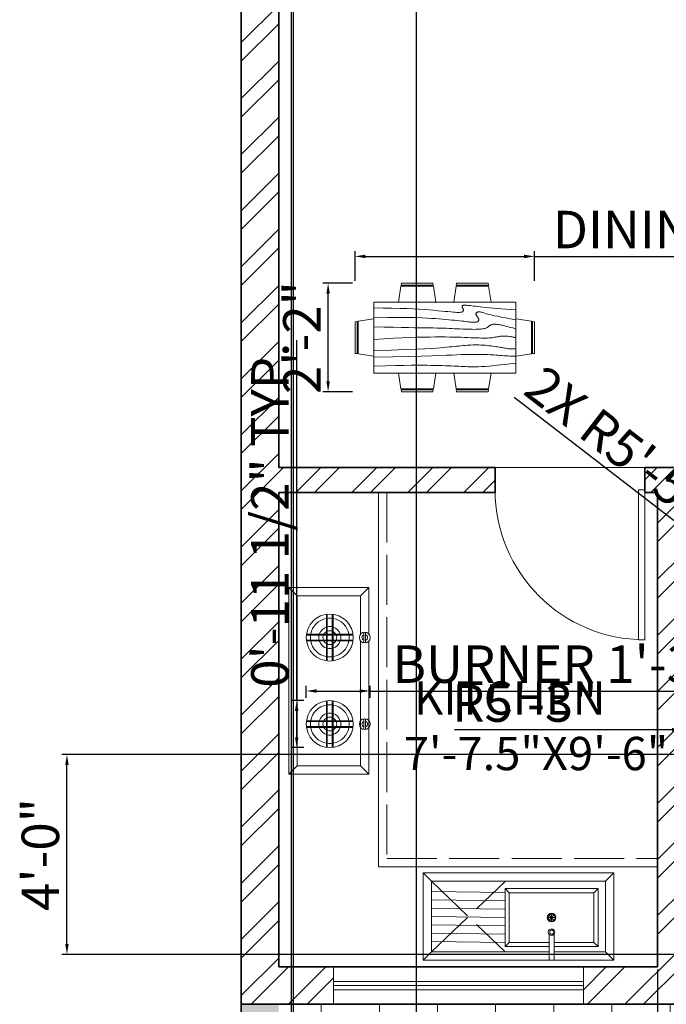
# Model space of a CAD drawing. Units: inches. Extents: x 287 to 905, y 1151 to 2037.
# Tile 2 of 5: x 361 to 516, y 1503 to 1739. Entities that reach past the tile are written whole.
import ezdxf

# ---------------------------------------------------------------- set-up
doc = ezdxf.new("R2010")
doc.units = ezdxf.units.IN
doc.linetypes.add('ACAD_ISO02W100', pattern=[15, 12, -3])
for name, color, linetype, lineweight in [('A-ANNO-DIMS', 2, 'Continuous', 18), ('A-AREA-IDEN', 7, 'Continuous', 18), ('A-DOOR', 4, 'Continuous', 18), ('A-EQPM', 8, 'Continuous', 18), ('A-FLOR-CASE', 8, 'Continuous', 18), ('A-FLOR-CASE-HIDN', 8, 'ACAD_ISO02W100', 13), ('A-FLOR-FIXT', 8, 'Continuous', 18), ('A-FLOR-FIXT-HIDN', 8, 'ACAD_ISO02W100', 13), ('A-FLOR-FIXT-PATT', 9, 'Continuous', 13), ('A-FLOR-PATT', 252, 'Continuous', 13), ('A-FURN', 9, 'Continuous', 18), ('A-WALL', 7, 'Continuous', 35), ('A-WALL-PATT', 252, 'Continuous', 13), ('L-WALL-PATT', 252, 'Continuous', 13)]:
    doc.layers.add(name, color=color, linetype=linetype, lineweight=lineweight)
doc.layers.add('A-GLAZ', color=244, linetype='Continuous', lineweight=18, true_color=0x991b1e)
doc.styles.get("Standard").update_dxf_attribs({"font": 'arial.ttf'})
doc.dimstyles.new('ISO-25', dxfattribs={"dimtxt": 9, "dimasz": 2.5, "dimexe": 1.25, "dimexo": 0.625, "dimtad": 1, "dimlunit": 3, "dimtxsty": 'Standard', "dimcen": 2.5, "dimadec": 0, "dimazin": 0, "dimtfac": 1, "dimtmove": 0, "dimatfit": 3, "dimfxl": 1, "dimarcsym": 0})

# ---------------------------------------------------------------- blocks, each defined once
blk = doc.blocks.new('*U6')
for p, q in [((0, 0), (0, -6)), ((40, 0), (40, -6))]:
    blk.add_line(p, q)
blk.add_lwpolyline([(0, 0), (0, 40), (1.75, 40), (1.75, 0)], close=True)
blk.add_arc((0, 0), 40, 0, 90)
blk = doc.blocks.new('Dining Set - 36 x 72 in.')
for p, q in [((-22.2343, 26.00059), (-23.4847, 17.99762)), ((-22.2304, 26), (-5.7608, 26)), ((-22, 27.5), (-22.1562, 26.50042)), ((-5.8416, 26.5), (-22.1534, 26.5)), ((-22, 27.5), (-6, 27.5)), ((-5.8437, 26.49966), (-6, 27.5)), ((-4.5152, 17.99762), (-5.7655, 25.99926)), ((5.7657, 26.00059), (4.5153, 17.99762)), ((5.7696, 26), (22.2392, 26)), ((6, 27.5), (5.8438, 26.50042)), ((22.1584, 26.5), (5.8466, 26.5)), ((6, 27.5), (22, 27.5)), ((22.1563, 26.49966), (22, 27.5)), ((23.4848, 17.99762), (22.2345, 25.99926)), ((36, 18), (-36, 18)), ((-36, 18), (-36, -18)), ((36, -18), (36, 18)), ((-45.5, 8), (-44.5004, 8.15617)), ((-45.5, 8), (-45.5, -8)), ((-44.5, -8.15843), (-44.5, 8.15338)), ((-44.0006, 8.23428), (-35.9976, 9.48474)), ((-44, 8.23041), (-44, -8.23915)), ((44.0006, 8.23428), (35.9976, 9.48474)), ((44, 8.23041), (44, -8.23915)), ((44.5, -8.15843), (44.5, 8.15338)), ((45.5, 8), (44.5005, 8.15617)), ((45.5, 8), (45.5, -8)), ((-44.4997, -8.15631), (-45.5, -8)), ((-35.9976, -9.48476), (-43.9993, -8.2345)), ((35.9976, -9.48476), (43.9993, -8.2345)), ((44.4997, -8.15631), (45.5, -8)), ((-36, -18), (36, -18)), ((-22.2343, -26.0006), (-23.4847, -17.99762)), ((-4.5152, -17.99762), (-5.7655, -25.99928)), ((5.7657, -26.0006), (4.5153, -17.99762)), ((23.4848, -17.99762), (22.2345, -25.99928)), ((-22.2304, -26), (-5.7608, -26)), ((-22, -27.5), (-22.1562, -26.50044)), ((-5.8416, -26.5), (-22.1534, -26.5)), ((-22, -27.5), (-6, -27.5)), ((-5.8437, -26.49967), (-6, -27.5)), ((5.7696, -26), (22.2392, -26)), ((6, -27.5), (5.8438, -26.50044)), ((22.1584, -26.5), (5.8466, -26.5)), ((6, -27.5), (22, -27.5)), ((22.1563, -26.49967), (22, -27.5))]:
    blk.add_line(p, q)
for points in [[(-36, 15), (-31.1772, 14.97754), (-26.8079, 14.91406), (-22.8538, 14.81543), (-19.276, 14.6875), (-16.0362, 14.53613), (-13.0957, 14.36718), (-10.4159, 14.18652), (-7.9583, 14), (-5.6904, 13.81315), (-3.6035, 13.63021), (-1.6954, 13.45508), (0.0365, 13.29166), (1.5945, 13.14388), (2.9811, 13.01562), (4.1988, 12.9108), (5.25, 12.83333), (6.1393, 12.78613), (6.8802, 12.76823), (7.4883, 12.77767), (7.9792, 12.8125), (8.3685, 12.87077), (8.6719, 12.95052), (8.9049, 13.0498), (9.0833, 13.16666), (9.2205, 13.29899), (9.3216, 13.44401), (9.3895, 13.59879), (9.4271, 13.76041), (9.4373, 13.92594), (9.4232, 14.09245), (9.3875, 14.257), (9.3333, 14.41666), (9.2638, 14.56917), (9.1836, 14.71484), (9.0975, 14.85465), (9.0104, 14.98958), (8.9272, 15.1206), (8.8529, 15.2487), (8.7922, 15.37483), (8.75, 15.5), (8.7305, 15.62467), (8.7344, 15.74739), (8.7617, 15.86621), (8.8125, 15.97916), (8.8867, 16.08431), (8.9844, 16.17968), (9.1055, 16.26334), (9.25, 16.33333), (9.4189, 16.38802), (9.6172, 16.42708), (9.8506, 16.45052), (10.125, 16.45833), (10.4463, 16.45052), (10.8203, 16.42708), (11.2529, 16.38802), (11.75, 16.33333), (12.3184, 16.26318), (12.9694, 16.17838), (13.7151, 16.07991), (14.5677, 15.96875), (15.5395, 15.84586), (16.6426, 15.71224), (17.8893, 15.56884), (19.2917, 15.41666), (20.859, 15.25667), (22.5879, 15.08984), (24.4721, 14.91715), (26.5052, 14.73958), (28.6809, 14.5581), (30.9929, 14.3737), (33.4347, 14.18733), (36, 14)], [(-36, 10), (-28.9766, 10.14274), (-23.1725, 10.20442), (-18.4241, 10.19775), (-14.5677, 10.13541), (-11.4399, 10.03011), (-8.877, 9.89453), (-6.7154, 9.74137), (-4.7917, 9.58333), (-2.9698, 9.43082), (-1.2246, 9.28515), (0.4415, 9.14534), (2.026, 9.01041), (3.5266, 8.87939), (4.9408, 8.7513), (6.266, 8.62516), (7.5, 8.5), (8.6411, 8.37549), (9.6914, 8.2539), (10.6538, 8.13818), (11.5312, 8.03125), (12.3267, 7.93603), (13.043, 7.85547), (13.6831, 7.79248), (14.25, 7.75), (14.7471, 7.7303), (15.1797, 7.73307), (15.5537, 7.75732), (15.875, 7.80208), (16.1494, 7.86637), (16.3828, 7.94922), (16.5811, 8.04964), (16.75, 8.16666), (16.8944, 8.29915), (17.0143, 8.44531), (17.1089, 8.60319), (17.1771, 8.77083), (17.218, 8.94629), (17.2305, 9.1276), (17.2137, 9.31282), (17.1667, 9.5), (17.0895, 9.6875), (16.987, 9.875), (16.8649, 10.0625), (16.7292, 10.25), (16.5856, 10.4375), (16.4401, 10.625), (16.2985, 10.8125), (16.1667, 11), (16.05, 11.18733), (15.9518, 11.3737), (15.8752, 11.5581), (15.8229, 11.73958), (15.798, 11.91715), (15.8034, 12.08984), (15.842, 12.25667), (15.9167, 12.41666), (16.0295, 12.56836), (16.1784, 12.70833), (16.3605, 12.83268), (16.5729, 12.9375), (16.8127, 13.01888), (17.0768, 13.07291), (17.3625, 13.0957), (17.6667, 13.08333), (17.9894, 13.03312), (18.3418, 12.94726), (18.7382, 12.82918), (19.1927, 12.68229), (19.7195, 12.51001), (20.3327, 12.31575), (21.0465, 12.10294), (21.875, 11.875), (22.8357, 11.63354), (23.959, 11.37304), (25.2786, 11.08618), (26.8282, 10.76562), (28.6414, 10.40405), (30.752, 9.99414), (33.1936, 9.52856), (36, 9)], [(-36, 5.5), (-30.7157, 5.3348), (-26.069, 5.20963), (-21.9946, 5.11767), (-18.4271, 5.05208), (-15.3009, 5.00602), (-12.5508, 4.97265), (-10.1112, 4.94515), (-7.9167, 4.91666), (-5.909, 4.88167), (-4.0586, 4.83984), (-2.3429, 4.79215), (-0.7396, 4.73958), (0.7739, 4.6831), (2.22, 4.6237), (3.6213, 4.56233), (5, 4.5), (6.373, 4.43782), (7.7344, 4.3776), (9.0723, 4.32129), (10.375, 4.27083), (11.6309, 4.22819), (12.8281, 4.19531), (13.9551, 4.17415), (15, 4.16666), (15.954, 4.17448), (16.819, 4.19791), (17.6001, 4.23698), (18.3021, 4.29166), (18.9299, 4.36198), (19.4883, 4.44791), (19.9823, 4.54948), (20.4167, 4.66666), (20.7969, 4.79899), (21.1302, 4.94401), (21.4245, 5.09879), (21.6875, 5.26041), (21.9271, 5.42594), (22.1511, 5.59245), (22.3672, 5.757), (22.5834, 5.91666), (22.8065, 6.06868), (23.0404, 6.21093), (23.2879, 6.34147), (23.5521, 6.45833), (23.8358, 6.55957), (24.142, 6.64323), (24.4735, 6.70735), (24.8334, 6.75), (25.2235, 6.76969), (25.642, 6.76692), (26.0858, 6.74267), (26.5521, 6.69791), (27.0379, 6.63362), (27.5404, 6.55078), (28.0565, 6.45036), (28.5834, 6.33333), (29.1242, 6.19987), (29.7071, 6.04687), (30.3661, 5.87044), (31.1354, 5.66666), (32.0493, 5.43164), (33.142, 5.16146), (34.4475, 4.85221), (36, 4.5)], [(-36, -1), (-30.7915, -0.6591), (-26.0195, -0.38216), (-21.6519, -0.16284), (-17.6563, 0.00521), (-14.0005, 0.12833), (-10.6523, 0.21289), (-7.5796, 0.26522), (-4.75, 0.29166), (-2.134, 0.29793), (0.2878, 0.28711), (2.5317, 0.26163), (4.6146, 0.22396), (6.5529, 0.17651), (8.3633, 0.12174), (10.0623, 0.06209), (11.6667, 0), (13.1899, -0.06201), (14.6341, -0.1211), (15.9982, -0.17432), (17.2813, -0.21875), (18.4823, -0.25147), (19.6003, -0.26953), (20.6343, -0.27002), (21.5834, -0.25), (22.4481, -0.20768), (23.2357, -0.14584), (23.9549, -0.06836), (24.6146, 0.02083), (25.2235, 0.11784), (25.7904, 0.21875), (26.3241, 0.31966), (26.8334, 0.41666), (27.3265, 0.50618), (27.8099, 0.58593), (28.2894, 0.65397), (28.7709, 0.70833), (29.2601, 0.74707), (29.763, 0.76823), (30.2855, 0.76985), (30.8334, 0.75), (31.4088, 0.70784), (31.9994, 0.64713), (32.589, 0.57275), (33.1615, 0.48958), (33.7008, 0.4025), (34.1908, 0.3164), (34.6153, 0.23616), (34.9584, 0.16666), (35.2099, 0.11165), (35.3848, 0.07031), (35.504, 0.04069), (35.5886, 0.02083), (35.6594, 0.00879), (35.7377, 0.0026), (35.8442, 0.00032), (36, 0)], [(-36, -6.5), (-27.1843, -6.31267), (-20.084, -6.1263), (-14.469, -5.9419), (-10.1094, -5.76042), (-6.7752, -5.58285), (-4.2363, -5.41016), (-2.2629, -5.24333), (-0.625, -5.08334), (0.8708, -4.93099), (2.2715, -4.78646), (3.5872, -4.64974), (4.8281, -4.52084), (6.0046, -4.39974), (7.127, -4.28646), (8.2053, -4.18099), (9.25, -4.08334), (10.2705, -3.99382), (11.2734, -3.91407), (12.2647, -3.84603), (13.25, -3.79167), (14.2354, -3.75293), (15.2266, -3.73177), (16.2295, -3.73015), (17.25, -3.75), (18.2912, -3.79248), (19.3451, -3.85547), (20.4009, -3.93604), (21.4479, -4.03125), (22.4754, -4.13819), (23.4727, -4.25391), (24.4289, -4.37549), (25.3334, -4.5), (26.1785, -4.62492), (26.9694, -4.74935), (27.7145, -4.87281), (28.4219, -4.99479), (29.1, -5.11483), (29.7572, -5.23242), (30.4016, -5.34709), (31.0417, -5.45834), (31.6837, -5.56437), (32.3262, -5.65821), (32.9658, -5.73153), (33.599, -5.77604), (34.2224, -5.78345), (34.8327, -5.74545), (35.4264, -5.65373), (36, -5.5)], [(-36, -10), (-26.4022, -9.81299), (-18.4675, -9.62891), (-11.9839, -9.45069), (-6.7396, -9.28125), (-2.5226, -9.12354), (0.8789, -8.98047), (3.6769, -8.85498), (6.0833, -8.75), (8.2767, -8.66765), (10.3021, -8.60677), (12.1712, -8.56543), (13.8958, -8.54167), (15.4876, -8.53353), (16.9583, -8.53907), (18.3197, -8.55632), (19.5834, -8.58334), (20.7616, -8.61841), (21.8685, -8.66081), (22.9188, -8.71004), (23.9271, -8.76563), (24.9081, -8.82707), (25.8763, -8.89388), (26.8465, -8.96558), (27.8334, -9.04167), (28.8474, -9.12118), (29.8828, -9.20117), (30.93, -9.27824), (31.9792, -9.34896), (33.0205, -9.40991), (34.0443, -9.45768), (35.0407, -9.48885), (36, -9.5)], [(-36, -14.5), (-30.0881, -14.33513), (-25.0332, -14.21224), (-20.7312, -14.12647), (-17.0781, -14.07292), (-13.97, -14.04671), (-11.3027, -14.04297), (-8.9724, -14.05681), (-6.875, -14.08334), (-4.9224, -14.11833), (-3.0905, -14.16016), (-1.3709, -14.20785), (0.2448, -14.26042), (1.7647, -14.3169), (3.1973, -14.3763), (4.5507, -14.43767), (5.8333, -14.5), (7.0554, -14.5621), (8.235, -14.62175), (9.3922, -14.67652), (10.5469, -14.72396), (11.7192, -14.76164), (12.929, -14.78711), (14.1965, -14.79794), (15.5417, -14.79167), (16.9933, -14.76424), (18.6152, -14.70508), (20.4804, -14.60197), (22.6615, -14.44271), (25.2312, -14.21509), (28.2624, -13.9069), (31.8277, -13.50594), (36, -13)]]:
    blk.add_lwpolyline(points)
blk = doc.blocks.new('WIN-60IN')
for p, q in [((-1, 30), (-1, -30)), ((0, 30), (0, -30)), ((1, 30), (1, -30))]:
    blk.add_line(p, q)
blk.add_lwpolyline([(-4.5, 30), (4.5, 30), (4.5, -30), (-4.5, -30)], close=True)
blk = doc.blocks.new('COOKTOP-BURNER-WITH-CONTROL')
for p, q in [((-0.8, 5.6), (-0.8, -5.6)), ((-0.6, 5.62), (-0.6, 0.8)), ((0.6, 5.62), (0.6, 0.8)), ((0.8, 5.6), (0.8, -5.6)), ((-5.62, 0.6), (-0.8, 0.6)), ((-5.6, 0.8), (5.6, 0.8)), ((-0.6, 0.6), (-0.6, -0.6)), ((-0.6, 0.6), (0.6, 0.6)), ((0.6, 0.6), (0.6, -0.6)), ((0.8, 0.6), (5.62, 0.6)), ((8.19, 1.27), (8.19, -1.27)), ((8.59, 1.27), (8.59, -1.27)), ((-5.62, -0.6), (-0.8, -0.6)), ((-5.6, -0.8), (5.6, -0.8)), ((-0.6, -0.6), (0.6, -0.6)), ((-0.6, -0.8), (-0.6, -5.62)), ((0.6, -0.8), (0.6, -5.62)), ((0.8, -0.6), (5.62, -0.6))]:
    blk.add_line(p, q)
for centre, radius in [((0, 0), 5.65), ((8.39, 0), 1.29)]:
    blk.add_circle(centre, radius)
for centre, radius, start, end in [((0, 0), 4.65, 99.901, 170.099), ((0, 0), 2.65, 107.5531, 162.4469), ((0, 0), 4.65, 82.5905, 97.4095), ((0, 0), 2.65, 76.927, 103.073), ((0, 0), 4.65, 9.901, 80.099), ((0, 0), 2.65, 17.5531, 72.4469), ((0, 0), 4.65, 172.5905, 187.4095), ((0, 0), 2.65, 166.927, 193.073), ((0, 0), 1.65, 158.7117, 201.2883), ((0, 0), 1.65, 118.9523, 151.0477), ((0, 0), 1.65, 68.7117, 111.2883), ((0, 0), 1.65, 28.9523, 61.0477), ((0, 0), 1.65, 338.7117, 21.2883), ((0, 0), 2.65, 346.927, 13.073), ((0, 0), 4.65, 352.5905, 7.4095), ((8.39, 0), 0.687, 106.9364, 253.0636), ((8.39, 0), 0.687, 286.9364, 73.0636), ((0, 0), 4.65, 189.901, 260.099), ((0, 0), 2.65, 197.5531, 252.4469), ((0, 0), 1.65, 208.9523, 241.0477), ((0, 0), 1.65, 248.7117, 291.2883), ((0, 0), 4.65, 279.901, 350.099), ((0, 0), 2.65, 287.5531, 342.4469), ((0, 0), 1.65, 298.9523, 331.0477), ((0, 0), 2.65, 256.927, 283.073), ((0, 0), 4.65, 262.5905, 277.4095)]:
    blk.add_arc(centre, radius, start, end)
blk = doc.blocks.new('*D26')
at = {"layer": 'A-ANNO-DIMS', "color": 0, "lineweight": -2, "transparency": 16777216}
for p, q in [((429.49, 1576.45), (429.49, 1579.37)), ((444.82, 1576.45), (444.82, 1579.37)), ((431.99, 1578.12), (442.32, 1578.12)), ((444.82, 1578.12), (580.58, 1578.12))]:
    blk.add_line(p, q, dxfattribs=at)
at = {"layer": 'A-ANNO-DIMS', "color": 0, "transparency": 16777216}
for points in [[(431.99, 1578.54), (431.99, 1577.71), (429.49, 1578.12)], [(442.32, 1578.54), (442.32, 1577.71), (444.82, 1578.12)]]:
    blk.add_solid(points, dxfattribs=at)
at = {"layer": 'Defpoints', "color": 0, "transparency": 16777216}
for p in [(429.49, 1575.83), (444.82, 1578.12), (444.82, 1575.83)]:
    blk.add_point(p, dxfattribs=at)
at = {"layer": 'A-ANNO-DIMS', "color": 0, "transparency": 16777216, "insert": (513.95, 1583.41), "char_height": 9, "attachment_point": 5}
blk.add_mtext('BURNER 1\'-3 1/2" TYP.', dxfattribs=at)
blk = doc.blocks.new('*D27')
at = {"layer": 'A-ANNO-DIMS', "color": 0, "lineweight": -2, "transparency": 16777216}
for p, q in [((427.19, 1575.83), (427.19, 1662.4)), ((428.86, 1575.83), (425.94, 1575.83)), ((427.19, 1567.02), (427.19, 1573.33)), ((428.86, 1564.52), (425.94, 1564.52))]:
    blk.add_line(p, q, dxfattribs=at)
at = {"layer": 'A-ANNO-DIMS', "color": 0, "transparency": 16777216}
for points in [[(426.77, 1573.33), (427.6, 1573.33), (427.19, 1575.83)], [(426.77, 1567.02), (427.6, 1567.02), (427.19, 1564.52)]]:
    blk.add_solid(points, dxfattribs=at)
at = {"layer": 'Defpoints', "color": 0, "transparency": 16777216}
for p in [(427.19, 1575.83), (429.49, 1575.83), (429.49, 1564.52)]:
    blk.add_point(p, dxfattribs=at)
at = {"layer": 'A-ANNO-DIMS', "color": 0, "transparency": 16777216, "insert": (421.91, 1620.36), "char_height": 9, "attachment_point": 5, "rotation": 90}
blk.add_mtext('0\'-11 1/2" TYP.', dxfattribs=at)
blk = doc.blocks.new('*D28')
at = {"layer": 'A-ANNO-DIMS', "color": 0, "lineweight": -2, "transparency": 16777216}
for p, q in [((441.2, 1676.71), (441.2, 1683.81)), ((443.7, 1682.56), (481.83, 1682.56)), ((484.33, 1676.71), (484.33, 1683.81)), ((484.33, 1682.56), (587, 1682.56))]:
    blk.add_line(p, q, dxfattribs=at)
at = {"layer": 'A-ANNO-DIMS', "color": 0, "transparency": 16777216}
for points in [[(443.7, 1682.97), (443.7, 1682.14), (441.2, 1682.56)], [(481.83, 1682.97), (481.83, 1682.14), (484.33, 1682.56)]]:
    blk.add_solid(points, dxfattribs=at)
at = {"layer": 'Defpoints', "color": 0, "transparency": 16777216}
for p in [(484.33, 1682.56), (441.2, 1676.09), (484.33, 1676.09)]:
    blk.add_point(p, dxfattribs=at)
at = {"layer": 'A-ANNO-DIMS', "color": 0, "transparency": 16777216, "insert": (536.92, 1687.84), "char_height": 9, "attachment_point": 5}
blk.add_mtext('DINING SET 3\'-7"', dxfattribs=at)
blk = doc.blocks.new('*D29')
at = {"layer": 'A-ANNO-DIMS', "color": 0, "lineweight": -2, "transparency": 16777216}
for p, q in [((440.58, 1676.09), (433.48, 1676.09)), ((434.73, 1652.52), (434.73, 1673.59)), ((440.58, 1650.02), (433.48, 1650.02))]:
    blk.add_line(p, q, dxfattribs=at)
at = {"layer": 'A-ANNO-DIMS', "color": 0, "transparency": 16777216}
for points in [[(434.32, 1673.59), (435.15, 1673.59), (434.73, 1676.09)], [(434.32, 1652.52), (435.15, 1652.52), (434.73, 1650.02)]]:
    blk.add_solid(points, dxfattribs=at)
at = {"layer": 'Defpoints', "color": 0, "transparency": 16777216}
for p in [(434.73, 1676.09), (441.2, 1676.09), (441.2, 1650.02)]:
    blk.add_point(p, dxfattribs=at)
at = {"layer": 'A-ANNO-DIMS', "color": 0, "transparency": 16777216, "insert": (429.59, 1663.05), "char_height": 9, "attachment_point": 5, "rotation": 90}
blk.add_mtext('2\'-2"', dxfattribs=at)
blk = doc.blocks.new('*D32')
at = {"layer": 'A-ANNO-DIMS', "color": 0, "lineweight": -2, "transparency": 16777216}
for p, q in [((426.39, 1284.46), (426.39, 2019.96)), ((428.89, 2018.71), (564.36, 2018.71)), ((566.86, 1284.46), (566.86, 2019.96))]:
    blk.add_line(p, q, dxfattribs=at)
at = {"layer": 'A-ANNO-DIMS', "color": 0, "transparency": 16777216}
for points in [[(428.89, 2019.12), (428.89, 2018.29), (426.39, 2018.71)], [(564.36, 2019.12), (564.36, 2018.29), (566.86, 2018.71)]]:
    blk.add_solid(points, dxfattribs=at)
at = {"layer": 'Defpoints', "color": 0, "transparency": 16777216}
for p in [(566.86, 2018.71), (426.39, 1283.83), (566.86, 1283.83)]:
    blk.add_point(p, dxfattribs=at)
at = {"layer": 'A-ANNO-DIMS', "color": 0, "transparency": 16777216, "insert": (496.62, 2023.99), "char_height": 9, "attachment_point": 5}
blk.add_mtext('11\'-8 1/2"', dxfattribs=at)
blk = doc.blocks.new('*D35')
at = {"layer": 'A-ANNO-DIMS', "color": 0, "lineweight": -2, "transparency": 16777216}
for p, q in [((651.73, 1562.83), (370.73, 1562.83)), ((371.98, 1517.33), (371.98, 1560.33)), ((651.73, 1514.83), (370.73, 1514.83))]:
    blk.add_line(p, q, dxfattribs=at)
at = {"layer": 'A-ANNO-DIMS', "color": 0, "transparency": 16777216}
for points in [[(371.57, 1560.33), (372.4, 1560.33), (371.98, 1562.83)], [(371.57, 1517.33), (372.4, 1517.33), (371.98, 1514.83)]]:
    blk.add_solid(points, dxfattribs=at)
at = {"layer": 'Defpoints', "color": 0, "transparency": 16777216}
for p in [(371.98, 1562.83), (652.36, 1562.83), (652.36, 1514.83)]:
    blk.add_point(p, dxfattribs=at)
at = {"layer": 'A-ANNO-DIMS', "color": 0, "transparency": 16777216, "insert": (366.76, 1538.83), "char_height": 9, "attachment_point": 5, "rotation": 90}
blk.add_mtext('4\'-0"', dxfattribs=at)
blk = doc.blocks.new('*D36')
at = {"layer": 'A-ANNO-DIMS', "color": 0, "lineweight": -2, "transparency": 16777216}
for p, q in [((513.86, 1511.21), (513.86, 1157.65)), ((519.86, 1511.21), (519.86, 1157.65)), ((511.36, 1158.9), (508.86, 1158.9)), ((513.86, 1158.9), (519.86, 1158.9)), ((522.36, 1158.9), (550.03, 1158.9))]:
    blk.add_line(p, q, dxfattribs=at)
at = {"layer": 'A-ANNO-DIMS', "color": 0, "transparency": 16777216}
for points in [[(511.36, 1159.32), (511.36, 1158.49), (513.86, 1158.9)], [(522.36, 1159.32), (522.36, 1158.49), (519.86, 1158.9)]]:
    blk.add_solid(points, dxfattribs=at)
at = {"layer": 'Defpoints', "color": 0, "transparency": 16777216}
for p in [(513.86, 1511.83), (519.86, 1511.83), (519.86, 1158.9)]:
    blk.add_point(p, dxfattribs=at)
at = {"layer": 'A-ANNO-DIMS', "color": 0, "transparency": 16777216, "insert": (537.44, 1164.12), "char_height": 9, "attachment_point": 5}
blk.add_mtext('0\'-6"', dxfattribs=at)
blk = doc.blocks.new('*D38')
at = {"layer": 'A-ANNO-DIMS', "color": 0, "lineweight": -2, "transparency": 16777216}
for p, q in [((425.86, 1913.21), (425.86, 1157.65)), ((455.86, 1913.21), (455.86, 1157.65)), ((428.36, 1158.9), (453.36, 1158.9))]:
    blk.add_line(p, q, dxfattribs=at)
at = {"layer": 'A-ANNO-DIMS', "color": 0, "transparency": 16777216}
for points in [[(428.36, 1159.32), (428.36, 1158.49), (425.86, 1158.9)], [(453.36, 1159.32), (453.36, 1158.49), (455.86, 1158.9)]]:
    blk.add_solid(points, dxfattribs=at)
at = {"layer": 'Defpoints', "color": 0, "transparency": 16777216}
for p in [(425.86, 1913.83), (455.86, 1913.83), (455.86, 1158.9)]:
    blk.add_point(p, dxfattribs=at)
at = {"layer": 'A-ANNO-DIMS', "color": 0, "transparency": 16777216, "insert": (440.86, 1164.12), "char_height": 9, "attachment_point": 5}
blk.add_mtext('2\'-6"', dxfattribs=at)
blk = doc.blocks.new('*D41')
at = {"layer": 'A-ANNO-DIMS', "color": 0, "lineweight": -2, "transparency": 16777216}
for p, q in [((479.4, 1648.76), (529.44, 1610.15)), ((582.98, 1568.83), (531.42, 1608.62))]:
    blk.add_line(p, q, dxfattribs=at)
at = {"layer": 'A-ANNO-DIMS', "color": 0, "transparency": 16777216}
blk.add_solid([(529.7, 1610.48), (529.19, 1609.82), (531.42, 1608.62)], dxfattribs=at)
at = {"layer": 'Defpoints', "color": 0, "transparency": 16777216}
for p in [(531.42, 1608.62), (582.98, 1568.83)]:
    blk.add_point(p, dxfattribs=at)
at = {"layer": 'A-ANNO-DIMS', "color": 0, "transparency": 16777216, "insert": (503.67, 1636.62), "char_height": 9, "attachment_point": 5, "rotation": 322.3456}
blk.add_mtext('2X R5\'-5"', dxfattribs=at)
blk = doc.blocks.new('*D42')
at = {"layer": 'A-ANNO-DIMS', "color": 0, "lineweight": -2, "transparency": 16777216}
for p, q in [((465.09, 1568.83), (517.36, 1568.83)), ((582.98, 1568.83), (519.86, 1568.83))]:
    blk.add_line(p, q, dxfattribs=at)
at = {"layer": 'A-ANNO-DIMS', "color": 0, "transparency": 16777216}
blk.add_solid([(517.36, 1569.25), (517.36, 1568.42), (519.86, 1568.83)], dxfattribs=at)
at = {"layer": 'Defpoints', "color": 0, "transparency": 16777216}
for p in [(519.86, 1568.83), (582.98, 1568.83)]:
    blk.add_point(p, dxfattribs=at)
at = {"layer": 'A-ANNO-DIMS', "color": 0, "transparency": 16777216, "insert": (481.98, 1574.06), "char_height": 9, "attachment_point": 5, "rotation": 0.0002}
blk.add_mtext('R5\'-3"', dxfattribs=at)

msp = doc.modelspace()

# ---------------------------------------------------------------- hatches: boundary and pattern name
at = {"layer": 'A-FLOR-FIXT-PATT'}
h = msp.add_hatch(dxfattribs=at)
h.set_pattern_fill('ANSI31', color=256, scale=0.6300798, angle=134.1764, style=0)
h.paths.add_polyline_path([(459.583, 1517.736), (477.272, 1517.482), (477.272, 1529.883), (459.583, 1530.137)])
at = {"layer": 'A-FLOR-PATT'}
h = msp.add_hatch(dxfattribs=at)
h.set_pattern_fill('ANGLE', color=256, scale=2)
h.set_pattern_definition([(0, (0, 0), (0, 13.97), [10.16, -3.81]), (90, (0, 0), (-13.97, 9e-16), [10.16, -3.81])])
h.paths.add_polyline_path([(588.313, 1502.833), (422.857, 1502.833), (422.857, 1283.833), (588.313, 1283.833)])
h.paths.add_polyline_path([(486.188, 1389.005), (563.901, 1389.005), (563.901, 1418.856), (486.188, 1418.856)], flags=24)
at = {"layer": 'A-WALL-PATT'}
h = msp.add_hatch(dxfattribs=at)
h.set_pattern_fill('ANSI32', color=256)
h.paths.add_polyline_path([(422.857, 1775.833), (561.857, 1775.833), (561.857, 1781.833), (568.629, 1788.605), (564.387, 1792.848), (553.372, 1781.833), (422.857, 1781.833), (422.857, 1913.833), (425.857, 1913.833), (425.857, 1919.833), (422.857, 1919.833), (422.857, 1967.833), (452.78, 1967.833), (452.78, 1976.833), (413.857, 1976.833), (413.857, 1502.833), (436.063, 1502.833), (436.063, 1511.833), (422.857, 1511.833), (422.857, 1625.833), (474.857, 1625.833), (474.857, 1631.833), (422.857, 1631.833)])
h = msp.add_hatch(dxfattribs=at)
h.set_pattern_fill('ANSI32', color=256)
h.paths.add_polyline_path([(604.357, 1511.833), (519.857, 1511.833), (519.857, 1625.833), (607.357, 1625.833), (607.357, 1631.833), (510.857, 1631.833), (510.857, 1625.833), (513.857, 1625.833), (513.857, 1511.833), (496.063, 1511.833), (496.063, 1502.833), (604.357, 1502.833)])
h.paths.add_polyline_path([(652.357, 1511.833), (652.357, 1514.833), (643.357, 1514.833), (643.357, 1511.833), (640.357, 1511.833), (640.357, 1505.833), (643.357, 1505.833), (643.357, 1370.833), (690.607, 1370.833), (690.607, 1379.833), (652.357, 1379.833)])
h.paths.add_polyline_path([(797.857, 1582.055), (788.857, 1582.055), (788.857, 1571.833), (703.357, 1571.833), (703.357, 1574.833), (697.357, 1574.833), (697.357, 1571.833), (652.357, 1571.833), (652.357, 1574.833), (646.357, 1574.833), (646.357, 1562.833), (652.357, 1562.833), (652.357, 1565.833), (788.857, 1565.833), (788.857, 1379.833), (750.607, 1379.833), (750.607, 1370.833), (797.857, 1370.833)])
h.paths.add_polyline_path([(797.857, 1673.833), (788.857, 1673.833), (788.857, 1631.833), (685.357, 1631.833), (685.357, 1625.833), (697.357, 1625.833), (697.357, 1604.833), (703.357, 1604.833), (703.357, 1625.833), (788.857, 1625.833), (788.857, 1603.055), (797.857, 1603.055)])
h.paths.add_polyline_path([(797.857, 1976.833), (751.357, 1976.833), (751.357, 1967.833), (788.857, 1967.833), (788.857, 1919.833), (785.857, 1919.833), (785.857, 1913.833), (788.857, 1913.833), (788.857, 1781.833), (654.342, 1781.833), (643.328, 1792.848), (639.085, 1788.605), (645.857, 1781.833), (645.857, 1775.833), (646.357, 1775.833), (646.357, 1772.833), (652.357, 1772.833), (652.357, 1775.833), (788.857, 1775.833), (788.857, 1733.833), (797.857, 1733.833)])
h.paths.add_polyline_path([(755.857, 1919.833), (692.857, 1919.833), (692.857, 1967.833), (730.357, 1967.833), (730.357, 1976.833), (473.78, 1976.833), (473.78, 1967.833), (518.857, 1967.833), (518.857, 1919.833), (455.857, 1919.833), (455.857, 1913.833), (567.857, 1913.833), (567.857, 1919.833), (524.857, 1919.833), (524.857, 1967.833), (686.857, 1967.833), (686.857, 1919.833), (639.857, 1919.833), (639.857, 1913.833), (755.857, 1913.833)])
h.paths.add_polyline_path([(606.857, 1913.833), (609.857, 1913.833), (609.857, 1919.833), (597.857, 1919.833), (597.857, 1913.833), (600.857, 1913.833), (600.857, 1829.319), (589.842, 1818.304), (594.085, 1814.061), (600.857, 1820.833), (600.857, 1781.833), (597.857, 1781.833), (597.857, 1775.833), (609.857, 1775.833), (609.857, 1781.833), (606.857, 1781.833), (606.857, 1820.833), (613.629, 1814.061), (617.872, 1818.304), (606.857, 1829.319)])
h.paths.add_polyline_path([(652.357, 1736.833), (646.357, 1736.833), (646.357, 1631.833), (643.357, 1631.833), (643.357, 1625.833), (646.357, 1625.833), (646.357, 1604.833), (652.357, 1604.833), (652.357, 1625.833), (655.357, 1625.833), (655.357, 1631.833), (652.357, 1631.833)])
at = {"layer": 'L-WALL-PATT'}
h = msp.add_hatch(color=256, dxfattribs=at)
h.dxf.hatch_style = 1
h.paths.add_polyline_path([(422.857, 1502.833), (413.857, 1502.833), (413.857, 1277.833), (426.388, 1277.833), (426.388, 1283.833), (422.857, 1283.833)])
h.paths.add_polyline_path([(644.857, 1283.833), (635.857, 1283.833), (635.857, 1277.833), (644.857, 1277.833)])
h.paths.add_polyline_path([(575.857, 1283.833), (566.857, 1283.833), (566.857, 1277.833), (575.857, 1277.833)])

# ---------------------------------------------------------------- linework, layer by layer
at = {"layer": 'A-DOOR'}
msp.add_line((510.857, 1631.833), (474.857, 1631.833), dxfattribs=at)
at = {"layer": 'A-EQPM'}
for p, q in [((427.324, 1601.014), (425.324, 1603.014)), ((442.531, 1601.014), (444.531, 1603.014)), ((427.324, 1560.115), (425.324, 1558.115)), ((442.531, 1560.115), (444.531, 1558.115))]:
    msp.add_line(p, q, dxfattribs=at)
for points in [[(444.531, 1590.148), (444.531, 1558.115), (425.324, 1558.115), (425.324, 1603.014), (444.531, 1603.014), (444.531, 1591.767)], [(442.531, 1590.148), (442.531, 1560.115), (427.324, 1560.115), (427.324, 1601.014), (442.531, 1601.014), (442.531, 1591.767)]]:
    msp.add_lwpolyline(points, dxfattribs=at)
at = {"layer": 'A-FLOR-CASE'}
for p, q in [((446.857, 1625.833), (446.857, 1535.833)), ((446.857, 1535.833), (513.857, 1535.833))]:
    msp.add_line(p, q, dxfattribs=at)
at = {"layer": 'A-FLOR-CASE-HIDN'}
for p, q in [((448.857, 1625.833), (448.857, 1537.833)), ((448.857, 1537.833), (513.857, 1537.833))]:
    msp.add_line(p, q, dxfattribs=at)
at = {"layer": 'A-FLOR-FIXT'}
for p, q in [((459.583, 1532.456), (457.583, 1534.456)), ((501.344, 1532.456), (503.344, 1534.456)), ((478.272, 1529.649), (477.272, 1530.649)), ((498.6, 1529.649), (499.6, 1530.649)), ((489.162, 1522.928), (487.71, 1524.437)), ((487.722, 1522.917), (489.15, 1524.448)), ((488.436, 1524.729), (488.436, 1522.636)), ((487.389, 1523.683), (489.483, 1523.683)), ((487.836, 1513.418), (487.836, 1519.657)), ((489.036, 1513.418), (489.036, 1519.657)), ((478.272, 1517.716), (477.272, 1516.716)), ((498.6, 1517.716), (499.6, 1516.716)), ((459.583, 1515.418), (457.583, 1513.418)), ((501.344, 1515.418), (503.344, 1513.418))]:
    msp.add_line(p, q, dxfattribs=at)
msp.add_lwpolyline([(457.583, 1534.456), (503.344, 1534.456), (503.344, 1513.418), (457.583, 1513.418)], close=True, dxfattribs=at)
for points in [[(487.836, 1515.418), (459.583, 1515.418), (459.583, 1532.456), (501.344, 1532.456), (501.344, 1515.418), (489.036, 1515.418)], [(489.036, 1516.716), (499.6, 1516.716), (499.6, 1530.649), (477.272, 1530.649), (477.272, 1516.716), (487.836, 1516.716)], [(489.036, 1517.716), (498.6, 1517.716), (498.6, 1529.649), (478.272, 1529.649), (478.272, 1517.716), (487.836, 1517.716)]]:
    msp.add_lwpolyline(points, dxfattribs=at)
for centre, radius in [((488.436, 1523.683), 1.047), ((488.436, 1523.683), 0.847), ((488.436, 1520.176), 0.793), ((488.436, 1520.176), 0.493)]:
    msp.add_circle(centre, radius, dxfattribs=at)
at = {"layer": 'A-FLOR-FIXT-HIDN'}
for p, q in [((459.583, 1532.456), (477.272, 1515.418)), ((459.583, 1515.418), (477.336, 1532.456))]:
    msp.add_line(p, q, dxfattribs=at)
at = {"layer": 'A-WALL'}
for p, q in [((413.857, 1976.833), (413.857, 1277.833)), ((422.857, 1775.833), (422.857, 1631.833)), ((422.857, 1631.833), (474.857, 1631.833)), ((474.857, 1625.833), (474.857, 1631.833)), ((510.857, 1625.833), (510.857, 1631.833)), ((510.857, 1631.833), (607.357, 1631.833)), ((422.857, 1625.833), (474.857, 1625.833)), ((422.857, 1625.833), (422.857, 1511.833)), ((510.857, 1625.833), (513.857, 1625.833)), ((513.857, 1625.833), (513.857, 1511.833)), ((422.857, 1511.833), (513.857, 1511.833)), ((413.857, 1502.833), (604.357, 1502.833))]:
    msp.add_line(p, q, dxfattribs=at)

# ---------------------------------------------------------------- block references
at = {"layer": 'A-DOOR', "xscale": 0.9000000000001479, "yscale": 0.9000000000001479, "zscale": 0.9000000000001479, "rotation": 180}
msp.add_blockref('*U6', (510.857, 1626.433), dxfattribs=at)
at = {"layer": 'A-EQPM'}
for p in [(435.139, 1590.957), (435.139, 1570.172)]:
    msp.add_blockref('COOKTOP-BURNER-WITH-CONTROL', p, dxfattribs=at)
at = {"layer": 'A-FURN', "xscale": 0.4739502964170205, "yscale": 0.4739502964170205, "zscale": 0.4739502964170205}
msp.add_blockref('Dining Set - 36 x 72 in.', (462.769, 1663.054), dxfattribs=at)
at = {"layer": 'A-GLAZ', "rotation": 89.99999999999969}
msp.add_blockref('WIN-60IN', (466.063, 1507.333), dxfattribs=at)

# ---------------------------------------------------------------- texts
at = {"layer": 'A-AREA-IDEN', "insert": (452.91, 1580.434), "char_height": 8, "attachment_point": 1}
msp.add_mtext_dynamic_manual_height_columns(' KITCHEN\\P7\'-7.5"X9\'-6"', width=60.9474, gutter_width=12.5, heights=[0], dxfattribs=at)

# ---------------------------------------------------------------- dimensions: what is measured, and where the dimension line sits
at = {"layer": 'A-ANNO-DIMS'}
for base, p1, p2, picture, middle in [((566.857, 2018.708), (426.388, 1283.833), (566.857, 1283.833), '*D32', (496.622, 2023.987)), ((455.857, 1158.902), (425.857, 1913.833), (455.857, 1913.833), '*D38', (440.857, 1164.122)), ((519.857, 1158.902), (513.857, 1511.833), (519.857, 1511.833), '*D36', (537.444, 1164.122))]:
    dim = msp.add_linear_dim(base=base, p1=p1, p2=p2, dimstyle='ISO-25', override={"dimdec": 1, "dimlfac": 1, "dimrnd": 0, "dimzin": 1, "dimdsep": 46, "dimlunit": 4, "dimfrac": 2}, dxfattribs=at)
    dim.commit()
    dim.dimension.update_dxf_attribs({"geometry": picture, "text_midpoint": middle})
for base, p1, p2, text, picture, middle in [((484.333, 1682.557), (441.204, 1676.088), (484.333, 1676.088), 'DINING SET <>', '*D28', (536.918, 1687.839)), ((444.817, 1578.125), (429.487, 1575.825), (444.817, 1575.825), 'BURNER <> TYP.', '*D26', (513.95, 1583.406))]:
    dim = msp.add_linear_dim(base=base, p1=p1, p2=p2, text=text, dimstyle='ISO-25', override={"dimdec": 1, "dimlfac": 1, "dimrnd": 0, "dimzin": 1, "dimdsep": 46, "dimlunit": 4, "dimfrac": 2}, dxfattribs=at)
    dim.commit()
    dim.dimension.update_dxf_attribs({"geometry": picture, "text_midpoint": middle})
for base, p1, p2, picture, middle in [((434.734, 1676.088), (441.204, 1650.021), (441.204, 1676.088), '*D29', (429.591, 1663.054)), ((371.982, 1562.833), (652.357, 1514.833), (652.357, 1562.833), '*D35', (366.762, 1538.833))]:
    dim = msp.add_linear_dim(base=base, p1=p1, p2=p2, angle=90, dimstyle='ISO-25', override={"dimdec": 1, "dimlfac": 1, "dimrnd": 0, "dimzin": 1, "dimdsep": 46, "dimlunit": 4, "dimfrac": 2}, dxfattribs=at)
    dim.commit()
    dim.dimension.update_dxf_attribs({"geometry": picture, "text_midpoint": middle})
dim = msp.add_linear_dim(base=(427.187, 1575.825), p1=(429.487, 1564.52), p2=(429.487, 1575.825), angle=90, text='<> TYP.', dimstyle='ISO-25', override={"dimdec": 1, "dimlfac": 1, "dimrnd": 0, "dimzin": 1, "dimdsep": 46, "dimlunit": 4, "dimfrac": 2}, dxfattribs=at)
dim.commit()
dim.dimension.update_dxf_attribs({"geometry": '*D27', "text_midpoint": (421.909, 1620.362)})
dim = msp.add_radius_dim(center=(582.982, 1568.833), mpoint=(531.422, 1608.618), text='2X <>', dimstyle='ISO-25', override={"dimdec": 1, "dimlfac": 1, "dimrnd": 0, "dimzin": 1, "dimdsep": 46, "dimlunit": 4, "dimfrac": 2}, dxfattribs=at)
dim.commit()
dim.dimension.update_dxf_attribs({"geometry": '*D41', "text_midpoint": (500.486, 1632.489), "dimtype": 164})
dim = msp.add_radius_dim(center=(582.982, 1568.833), mpoint=(519.857, 1568.833), dimstyle='ISO-25', override={"dimdec": 1, "dimlfac": 1, "dimrnd": 0, "dimzin": 1, "dimdsep": 46, "dimlunit": 4, "dimfrac": 2}, dxfattribs=at)
dim.commit()
dim.dimension.update_dxf_attribs({"geometry": '*D42', "text_midpoint": (481.982, 1568.833), "dimtype": 164})

doc.saveas('drawing.dxf')
